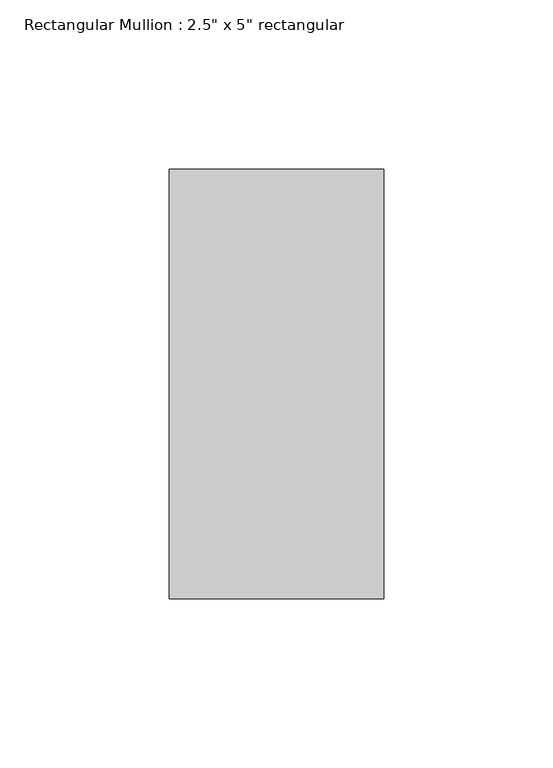
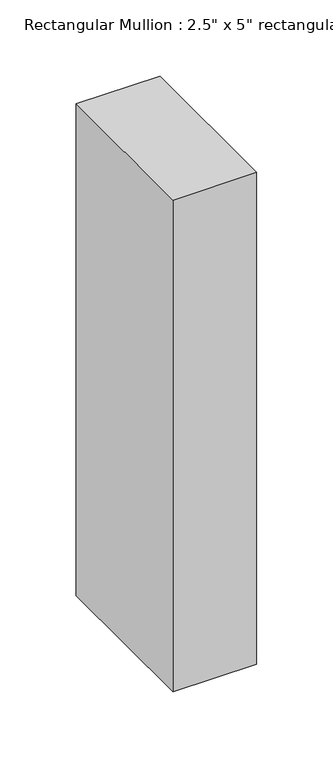
"""IFC4 building model written with IfcOpenShell, lengths in millimetres: member geometry."""

from ifc_helpers import new_model, si_unit, frame, origin, place, context, project, spatial, polyline, outline, extrude, source, transform, mapped, element, save


def member_7096a90e(model_context):
    return source(origin(), model_context, "Body", "SweptSolid", [
        extrude(outline(polyline([(0.0, 63.5), (0.0, -63.5), (-63.5, -63.5), (-63.5, 63.5), (0.0, 63.5)])), frame((0.0, 0.0, -393.7), z_axis=(0.0, 0.0, 1.0), x_axis=(1.0, 0.0, 0.0)), (0.0, 0.0, 1.0), 393.7),
    ])


if __name__ == "__main__":
    model = new_model("IFC4")
    model_context = context("Model", 3, world=origin())
    ifc_project = project(units=[si_unit("LENGTHUNIT", "METRE", prefix="MILLI")], contexts=[model_context])
    site = spatial("IfcSite", under=ifc_project)
    building = spatial("IfcBuilding", under=site)
    placement = place(None, origin())
    member_shape = member_7096a90e(model_context)
    element("IfcMember", 1, ObjectType="Rectangular Mullion : 2.5\" x 5\" rectangular", at=placement, inside=building, context=model_context, shape_type="MappedRepresentation", body=[
        mapped(member_shape, transform((0.0, 0.0, 0.0), x_axis=(1.0, 0.0, 0.0), y_axis=(0.0, 1.0, 0.0), z_axis=(0.0, 0.0, 1.0))),
    ])
    save(model, "model.ifc")

# Revit data of these elements
# Type "Rectangular Mullion : 2.5\" x 5\" rectangular"
#   built-in parameter 1007304 = 0.416667 (stored number, unit not read)
#   built-in parameter 1007301 = 0.104167 (stored number, unit not read)
#   built-in parameter 1007300 = 0.104167 (stored number, unit not read)
